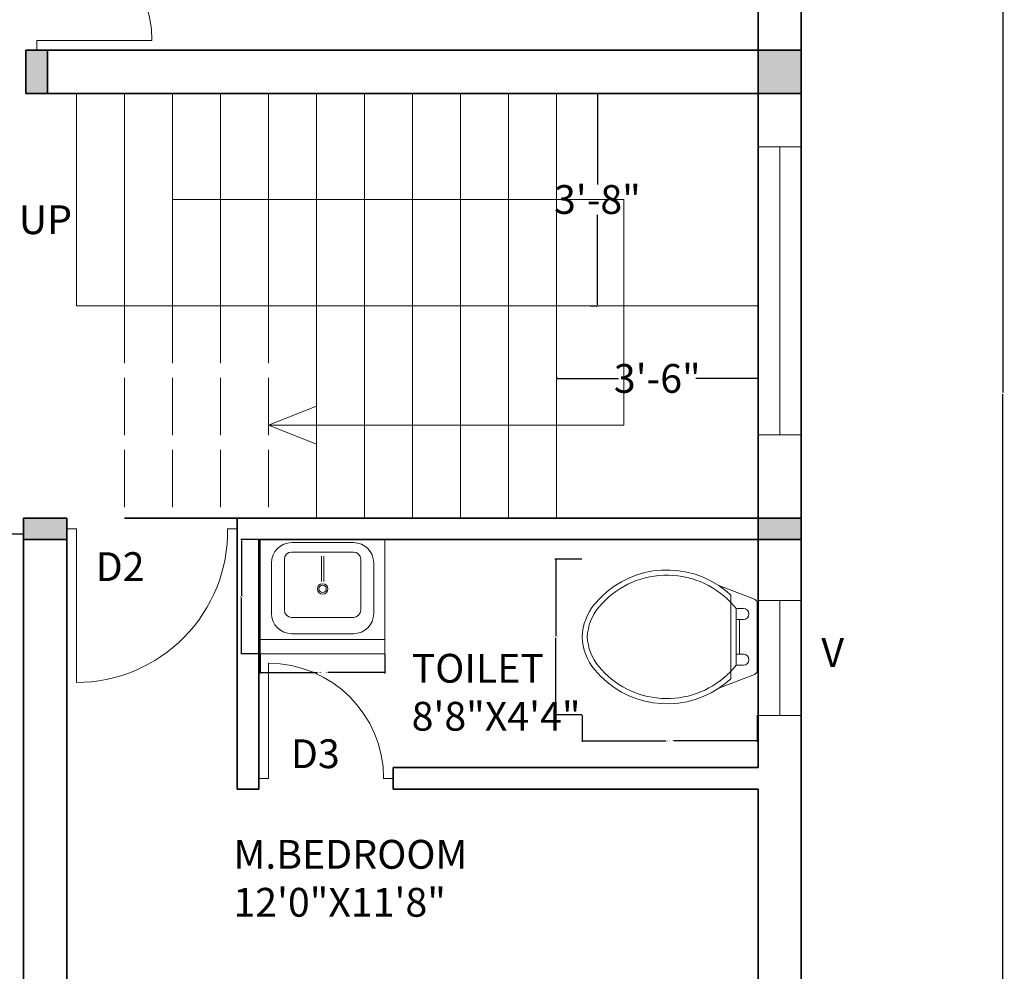
# Model space of a CAD drawing. Units: inches. Extents: x -36302355 to 648, y -221479757 to 75.
# Tile 22 of 37: x 442 to 647, y -469 to -271. Entities that reach past the tile are written whole.
import ezdxf

# ---------------------------------------------------------------- set-up
doc = ezdxf.new("R2010")
doc.units = ezdxf.units.IN
doc.header["$MEASUREMENT"] = 0
doc.linetypes.add('ACAD_ISO02W100', pattern=[15, 12, -3])
for name, color, linetype, lineweight in [('A-ANNO-DIMS', 2, 'Continuous', 18), ('A-ANNO-IDEN', 7, 'Continuous', 18), ('A-ANNO-TEXT', 7, 'Continuous', 18), ('A-AREA-IDEN', 7, 'Continuous', 18), ('A-COLS', 7, 'Continuous', 35), ('A-COLS-PATT', 242, 'Continuous', 13), ('A-DOOR', 4, 'Continuous', 18), ('A-FLOR-FIXT', 9, 'Continuous', 18), ('A-FLOR-STRS', 7, 'Continuous', 18), ('A-FLOR-STRS-HIDN', 7, 'ACAD_ISO02W100', 13), ('A-GLAZ', 142, 'Continuous', 18), ('A-WALL', 7, 'Continuous', 35)]:
    doc.layers.add(name, color=color, linetype=linetype, lineweight=lineweight)
doc.styles.get("Standard").update_dxf_attribs({"font": 'arial.ttf'})
doc.dimstyles.get("Standard").update_dxf_attribs({"dimtxt": 0.18, "dimasz": 0.18, "dimexe": 0.18, "dimexo": 0.0625, "dimgap": 0.09, "dimtad": 0, "dimtih": 1, "dimtoh": 1, "dimdec": 0, "dimzin": 0, "dimdsep": 46, "dimlunit": 3, "dimtxsty": 'Standard', "dimcen": 0.09, "dimadec": 0, "dimazin": 0, "dimtfac": 1, "dimtdec": 0, "dimtofl": 0, "dimtmove": 0, "dimatfit": 3, "dimfxl": 1, "dimtolj": 1, "dimtzin": 0, "dimarcsym": 0})

# ---------------------------------------------------------------- blocks, each defined once
blk = doc.blocks.new('*D5')
at = {"layer": 'A-ANNO-DIMS', "color": 0, "lineweight": -2, "transparency": 16777216}
for p, q in [((401.2, -376.83), (401.2, -378.08)), ((443.2, -376.83), (443.2, -378.08)), ((401.38, -377.9), (414.13, -377.9)), ((443.02, -377.9), (430.26, -377.9))]:
    blk.add_line(p, q, dxfattribs=at)
at = {"layer": 'A-ANNO-DIMS', "color": 0, "transparency": 16777216}
for points in [[(401.38, -377.87), (401.38, -377.93), (401.2, -377.9)], [(443.02, -377.87), (443.02, -377.93), (443.2, -377.9)]]:
    blk.add_solid(points, dxfattribs=at)
at = {"layer": 'Defpoints', "color": 0, "transparency": 16777216}
for p in [(401.2, -376.77), (443.2, -376.77), (443.2, -377.9)]:
    blk.add_point(p, dxfattribs=at)
at = {"layer": 'A-ANNO-DIMS', "color": 0, "transparency": 16777216, "insert": (422.2, -377.9), "char_height": 6, "attachment_point": 5}
blk.add_mtext('\\A1;3\'-6"', dxfattribs=at)
blk = doc.blocks.new('М14 600х655')
for p, q in [((-655, 600), (-655, 0)), ((-655, 600), (-655, 0)), ((-655, 0), (-655, 600)), ((0, 600), (-655, 600)), ((0, 0), (0, 600)), ((0, 525), (-655, 525)), ((-165.1, 494.1), (-489.9, 494.1)), ((-595.8, 388.1), (-595.8, 121.3)), ((-528.4, 370.1), (-528.4, 103.3)), ((-165.4, 408.4), (-490.2, 408.4)), ((-127.2, 103.3), (-127.2, 370.1)), ((-59.2, 121.3), (-59.2, 388.1)), ((-333.5, 87.1), (-333.5, 219.6)), ((-321.5, 87.1), (-321.5, 219.6)), ((-490.2, 65.1), (-165.4, 65.1)), ((-655, 0), (-655, 0)), ((-655, 0), (-655, 0)), ((-655, 0), (0, 0)), ((-655, 0), (0, 0)), ((-489.9, 15.4), (-165.1, 15.4))]:
    blk.add_line(p, q)
for radius in [27.6, 19.3]:
    blk.add_circle((-327.5, 258.9), radius)
for centre, radius, start, end in [((-489.9, 388.1), 105.9, 90, 180), ((-165.1, 388.1), 105.9, 0, 90), ((-490.2, 370.1), 38.2, 90, 180), ((-165.4, 370.1), 38.2, 0, 90), ((-489.9, 121.3), 105.9, 180, 270), ((-165.1, 121.3), 105.9, 270, 0), ((-490.2, 103.3), 38.2, 180, 270), ((-165.4, 103.3), 38.2, 270, 0)]:
    blk.add_arc(centre, radius, start, end)
blk = doc.blocks.new('*D13')
at = {"layer": 'A-ANNO-DIMS', "color": 0, "lineweight": -2, "transparency": 16777216}
for p, q in [((554.2, -345.07), (554.2, -345.6)), ((554.38, -345.42), (567.13, -345.42)), ((596.02, -345.42), (583.26, -345.42)), ((596.2, -345.07), (596.2, -345.6))]:
    blk.add_line(p, q, dxfattribs=at)
at = {"layer": 'A-ANNO-DIMS', "color": 0, "transparency": 16777216}
for points in [[(554.38, -345.39), (554.38, -345.45), (554.2, -345.42)], [(596.02, -345.39), (596.02, -345.45), (596.2, -345.42)]]:
    blk.add_solid(points, dxfattribs=at)
at = {"layer": 'Defpoints', "color": 0, "transparency": 16777216}
for p in [(554.2, -345.01), (596.2, -345.01), (596.2, -345.42)]:
    blk.add_point(p, dxfattribs=at)
at = {"layer": 'A-ANNO-DIMS', "color": 0, "transparency": 16777216, "insert": (575.2, -345.42), "char_height": 6, "attachment_point": 5}
blk.add_mtext('\\A1;3\'-6"', dxfattribs=at)
blk = doc.blocks.new('*D14')
at = {"layer": 'A-ANNO-DIMS', "color": 0, "lineweight": -2, "transparency": 16777216}
for p, q in [((561.2, -286.02), (562.91, -286.02)), ((562.73, -286.2), (562.73, -304.99)), ((562.73, -330.09), (562.73, -311.3)), ((561.2, -330.27), (562.91, -330.27))]:
    blk.add_line(p, q, dxfattribs=at)
at = {"layer": 'A-ANNO-DIMS', "color": 0, "transparency": 16777216}
for points in [[(562.7, -286.2), (562.76, -286.2), (562.73, -286.02)], [(562.7, -330.09), (562.76, -330.09), (562.73, -330.27)]]:
    blk.add_solid(points, dxfattribs=at)
at = {"layer": 'Defpoints', "color": 0, "transparency": 16777216}
for p in [(561.14, -286.02), (562.73, -286.02), (561.14, -330.27)]:
    blk.add_point(p, dxfattribs=at)
at = {"layer": 'A-ANNO-DIMS', "color": 0, "transparency": 16777216, "insert": (562.73, -308.14), "char_height": 6, "attachment_point": 5}
blk.add_mtext('\\A1;3\'-8"', dxfattribs=at)
blk = doc.blocks.new('WC-FLOOR-MOUNT')
for p, q in [((4.02, 15.38), (4.02, 16.49)), ((4.02, 15.38), (4.02, 10.15)), ((4.02, 4.92), (4.02, 10.15)), ((4.02, 3.8), (4.02, 4.92))]:
    blk.add_line(p, q)
for points in [[(4.02, 15.38, -0.448546), (24.05, 14.64, -0.162618), (25.78, 10.15, -0.470877)], [(5.85, 17.93, -0.383919), (24.66, 15.14, -0.163732), (26.58, 10.15, -0.359733)], [(0, 10.15), (0, 15.22, -0.31031), (0.43, 15.85), (5.85, 17.93, -0.209071)], [(4.02, 16.49, -0.040937), (5.85, 17.93, -0.163732)], [(3.22, 14.46, -0.022712), (4.02, 15.38, -0.162618)], [(3.22, 14.46), (2.11, 14.46, 1), (2.11, 12.77), (2.69, 12.77)], [(3.22, 10.15), (3.22, 14.46, -0.476108)], [(0, 10.15), (0, 5.07, 0.31031), (0.43, 4.45), (5.85, 2.37, 0.209071)], [(3.22, 10.15), (3.22, 5.84, 0.022712)], [(4.57, 4.39, 0.431639), (24.05, 5.66, 0.162618), (25.78, 10.15, 0.470877)], [(5.85, 2.37, 0.383919), (24.66, 5.15, 0.163732), (26.58, 10.15, 0.359733)], [(3.22, 5.84), (2.11, 5.84, -1), (2.11, 7.53), (2.69, 7.53)], [(3.22, 5.84, 0.022712), (4.02, 4.92, 0.162618)], [(4.02, 4.92, 0.014165), (4.57, 4.39, 0.162618)], [(4.02, 3.8, 0.040937), (5.85, 2.37, 0.163732)]]:
    blk.add_lwpolyline(points, format="xyb")
for points in [[(2.69, 12.77), (2.69, 7.53)], [(2.69, 12.77), (3.22, 12.77)], [(2.69, 7.53), (3.22, 7.53)]]:
    blk.add_lwpolyline(points)
blk = doc.blocks.new('WIN-60')
for p, q in [((60, 9), (0, 9)), ((0, 9), (0, 0)), ((60, 0), (60, 9)), ((0, 4.5), (60, 4.5)), ((0, 0), (60, 0))]:
    blk.add_line(p, q)
blk = doc.blocks.new('VENT-24')
for p, q in [((0, 0), (0, 24)), ((0, 24), (9, 24)), ((4.5, 24), (4.5, 0)), ((9, 24), (9, 0)), ((9, 0), (0, 0))]:
    blk.add_line(p, q)
blk = doc.blocks.new('DOOR-SWING-24')
for p, q in [((0, 26), (0, 28)), ((0, 0), (0, 2)), ((0, 2), (24, 2))]:
    blk.add_line(p, q)
blk.add_arc((0, 2), 24, 0, 90)
blk = doc.blocks.new('*D29')
at = {"layer": 'A-ANNO-DIMS', "color": 0, "lineweight": -2, "transparency": 16777216}
for p, q in [((492.52, -402.87), (492.52, -406.88)), ((518.48, -402.87), (518.48, -406.88)), ((492.7, -406.7), (504.45, -406.7)), ((518.3, -406.7), (506.55, -406.7))]:
    blk.add_line(p, q, dxfattribs=at)
at = {"layer": 'A-ANNO-DIMS', "color": 0, "transparency": 16777216}
for points in [[(492.7, -406.67), (492.7, -406.73), (492.52, -406.7)], [(518.3, -406.67), (518.3, -406.73), (518.48, -406.7)]]:
    blk.add_solid(points, dxfattribs=at)
at = {"layer": 'Defpoints', "color": 0, "transparency": 16777216}
for p in [(492.52, -402.81), (518.48, -402.81), (518.48, -406.7)]:
    blk.add_point(p, dxfattribs=at)
at = {"layer": 'A-ANNO-DIMS', "color": 0, "transparency": 16777216, "insert": (505.5, -406.7), "char_height": 0.18, "attachment_point": 5}
blk.add_mtext('\\A1;BASIN 2\'-2" TYP.', dxfattribs=at)
blk = doc.blocks.new('*D30')
at = {"layer": 'A-ANNO-DIMS', "color": 0, "lineweight": -2, "transparency": 16777216}
for p, q in [((492.45, -379.02), (488.44, -379.02)), ((488.62, -379.2), (488.62, -390.73)), ((488.62, -402.63), (488.62, -391.09)), ((492.45, -402.81), (488.44, -402.81))]:
    blk.add_line(p, q, dxfattribs=at)
at = {"layer": 'A-ANNO-DIMS', "color": 0, "transparency": 16777216}
for points in [[(488.59, -379.2), (488.65, -379.2), (488.62, -379.02)], [(488.59, -402.63), (488.65, -402.63), (488.62, -402.81)]]:
    blk.add_solid(points, dxfattribs=at)
at = {"layer": 'Defpoints', "color": 0, "transparency": 16777216}
for p in [(492.52, -379.02), (488.62, -402.81), (492.52, -402.81)]:
    blk.add_point(p, dxfattribs=at)
at = {"layer": 'A-ANNO-DIMS', "color": 0, "transparency": 16777216, "insert": (488.62, -390.91), "char_height": 0.18, "attachment_point": 5}
blk.add_mtext('\\A1;2\'-0" TYP.', dxfattribs=at)
blk = doc.blocks.new('*D41')
at = {"layer": 'A-ANNO-DIMS', "color": 0, "lineweight": -2, "transparency": 16777216}
for p, q in [((559.53, -415.56), (559.53, -421.15)), ((596.04, -415.56), (596.04, -421.15)), ((559.71, -420.97), (577, -420.97)), ((595.86, -420.97), (578.57, -420.97))]:
    blk.add_line(p, q, dxfattribs=at)
at = {"layer": 'A-ANNO-DIMS', "color": 0, "transparency": 16777216}
for points in [[(559.71, -420.94), (559.71, -421), (559.53, -420.97)], [(595.86, -420.94), (595.86, -421), (596.04, -420.97)]]:
    blk.add_solid(points, dxfattribs=at)
at = {"layer": 'Defpoints', "color": 0, "transparency": 16777216}
for p in [(559.53, -415.5), (596.04, -415.5), (559.53, -420.97)]:
    blk.add_point(p, dxfattribs=at)
at = {"layer": 'A-ANNO-DIMS', "color": 0, "transparency": 16777216, "insert": (577.78, -420.97), "char_height": 0.18, "attachment_point": 5}
blk.add_mtext('\\A1;WC 3\'-0 1/2"', dxfattribs=at)
blk = doc.blocks.new('*D42')
at = {"layer": 'A-ANNO-DIMS', "color": 0, "lineweight": -2, "transparency": 16777216}
for p, q in [((559.47, -383.06), (553.87, -383.06)), ((554.05, -383.24), (554.05, -399.1)), ((554.05, -415.32), (554.05, -399.46)), ((559.47, -415.5), (553.87, -415.5))]:
    blk.add_line(p, q, dxfattribs=at)
at = {"layer": 'A-ANNO-DIMS', "color": 0, "transparency": 16777216}
for points in [[(554.02, -383.24), (554.08, -383.24), (554.05, -383.06)], [(554.02, -415.32), (554.08, -415.32), (554.05, -415.5)]]:
    blk.add_solid(points, dxfattribs=at)
at = {"layer": 'Defpoints', "color": 0, "transparency": 16777216}
for p in [(554.05, -383.06), (559.53, -383.06), (559.53, -415.5)]:
    blk.add_point(p, dxfattribs=at)
at = {"layer": 'A-ANNO-DIMS', "color": 0, "transparency": 16777216, "insert": (554.05, -399.28), "char_height": 0.18, "attachment_point": 5}
blk.add_mtext('\\A1;2\'-8 1/2"', dxfattribs=at)
blk = doc.blocks.new('*D57')
at = {"layer": 'A-ANNO-DIMS', "color": 0, "lineweight": -2, "transparency": 16777216}
for p, q in [((605.26, 24.98), (647.33, 24.98)), ((647.15, 24.8), (647.15, -348.34)), ((647.15, -721.84), (647.15, -348.7)), ((605.26, -722.02), (647.33, -722.02))]:
    blk.add_line(p, q, dxfattribs=at)
at = {"layer": 'A-ANNO-DIMS', "color": 0, "transparency": 16777216}
for points in [[(647.12, 24.8), (647.18, 24.8), (647.15, 24.98)], [(647.12, -721.84), (647.18, -721.84), (647.15, -722.02)]]:
    blk.add_solid(points, dxfattribs=at)
at = {"layer": 'Defpoints', "color": 0, "transparency": 16777216}
for p in [(605.2, 24.98), (605.2, -722.02), (647.15, -722.02)]:
    blk.add_point(p, dxfattribs=at)
at = {"layer": 'A-ANNO-DIMS', "color": 0, "transparency": 16777216, "insert": (647.15, -348.52), "char_height": 0.18, "attachment_point": 5}
blk.add_mtext('\\A1;62\'-3"', dxfattribs=at)

msp = doc.modelspace()

# ---------------------------------------------------------------- hatches: boundary and pattern name
at = {"layer": 'A-COLS-PATT'}
h = msp.add_hatch(color=256, dxfattribs=at)
h.dxf.hatch_style = 1
h.paths.add_polyline_path([(145.2, 24.98), (145.2, 15.98), (154.2, 15.98), (154.2, 24.98)])
h.paths.add_polyline_path([(247.2, 15.98), (247.2, 24.98), (238.2, 24.98), (238.2, 15.98)])
h.paths.add_polyline_path([(387.64, 15.98), (395.7, 15.98), (395.7, 24.98), (387.64, 24.98)])
h.paths.add_polyline_path([(451.26, 24.98), (443.7, 24.98), (443.7, 15.98), (451.26, 15.98)])
h.paths.add_polyline_path([(596.2, 15.98), (605.2, 15.98), (605.2, 24.98), (596.2, 24.98)])
h.paths.add_polyline_path([(238.2, -122.02), (238.2, -131.02), (247.2, -131.02), (247.2, -122.02)])
h.paths.add_polyline_path([(395.7, -122.02), (387.46, -122.02), (387.46, -131.02), (395.7, -131.02)])
h.paths.add_polyline_path([(448.2, -131.02), (453.73, -131.02), (453.73, -122.02), (443.7, -122.02), (443.7, -131.02)])
h.paths.add_polyline_path([(596.2, -131.02), (605.2, -131.02), (605.2, -122.02), (596.2, -122.02)])
h.paths.add_polyline_path([(145.2, -176.97), (154.2, -176.97), (154.2, -167.02), (145.2, -167.02)])
h.paths.add_polyline_path([(314.2, -176.97), (323.2, -176.97), (323.2, -167.02), (314.2, -167.02)])
h.paths.add_polyline_path([(154.2, -314.02), (154.2, -309.52), (145.2, -309.52), (145.2, -314.02)])
h.paths.add_polyline_path([(314.2, -309.52), (314.2, -318.52), (323.2, -318.52), (323.2, -309.52)])
h.paths.add_polyline_path([(448.2, -277.02), (443.7, -277.02), (443.7, -286.02), (448.2, -286.02)])
h.paths.add_polyline_path([(283.2, -370.02), (274.2, -370.02), (274.2, -379.02), (283.2, -379.02), (283.2, -374.52)])
h.paths.add_polyline_path([(154.2, -370.02), (145.2, -370.02), (145.2, -379.02), (154.2, -379.02)])
h.paths.add_polyline_path([(443.2, -374.52), (443.2, -379.02), (452.2, -379.02), (452.2, -374.52)])
h.paths.add_polyline_path([(145.2, -580.02), (154.2, -580.02), (154.2, -571.02), (145.2, -571.02)])
h.paths.add_polyline_path([(274.2, -571.02), (274.2, -580.02), (283.2, -580.02), (283.2, -571.02)])
h.paths.add_polyline_path([(443.2, -580.02), (452.2, -580.02), (452.2, -571.02), (443.2, -571.02)])
h = msp.add_hatch(color=256, dxfattribs=at)
h.dxf.hatch_style = 1
h.paths.add_polyline_path([(596.2, -277.02), (596.2, -286.02), (605.2, -286.02), (605.2, -277.02)])
h = msp.add_hatch(color=256, dxfattribs=at)
h.dxf.hatch_style = 1
h.paths.add_polyline_path([(605.2, -571.02), (596.2, -571.02), (596.2, -580.02), (605.2, -580.02)])
h.paths.add_polyline_path([(605.2, -374.52), (596.2, -374.52), (596.2, -379.02), (605.2, -379.02)])

# ---------------------------------------------------------------- linework, layer by layer
at = {"layer": 'A-COLS'}
for p, q in [((443.7, -277.02), (443.7, -286.02)), ((448.2, -277.02), (448.2, -286.02)), ((443.2, -374.52), (452.2, -374.52)), ((443.2, -379.02), (452.2, -379.02))]:
    msp.add_line(p, q, dxfattribs=at)
at = {"layer": 'A-DOOR'}
for p, q in [((452.2, -376.77), (454.2, -376.77)), ((454.2, -376.77), (454.2, -408.77)), ((487.7, -376.77), (485.7, -376.77))]:
    msp.add_line(p, q, dxfattribs=at)
msp.add_arc((454.2, -377.27), 31.5, 270, 0.9023, dxfattribs=at)
at = {"layer": 'A-FLOR-STRS'}
for p, q in [((454.2, -286.02), (454.2, -330.27)), ((464.2, -286.02), (464.2, -330.27)), ((474.2, -286.02), (474.2, -330.27)), ((484.2, -286.02), (484.2, -330.27)), ((494.2, -286.02), (494.2, -330.27)), ((504.2, -286.02), (504.2, -374.52)), ((514.2, -286.02), (514.2, -374.52)), ((524.2, -286.02), (524.2, -374.52)), ((534.2, -286.02), (534.2, -374.52)), ((544.2, -286.02), (544.2, -374.52)), ((554.2, -286.02), (554.2, -374.52)), ((474.2, -308.14), (568.21, -308.14)), ((568.21, -308.14), (568.21, -355.15)), ((454.2, -330.27), (596.2, -330.27)), ((494.2, -355.15), (504.2, -351.19)), ((568.21, -355.15), (494.2, -355.15)), ((494.2, -355.15), (504.2, -359.11))]:
    msp.add_line(p, q, dxfattribs=at)
at = {"layer": 'A-FLOR-STRS-HIDN'}
for p, q in [((464.2, -330.27), (464.2, -374.52)), ((474.2, -330.27), (474.2, -374.52)), ((484.2, -330.27), (484.2, -374.52)), ((494.2, -330.27), (494.2, -374.52))]:
    msp.add_line(p, q, dxfattribs=at)
at = {"layer": 'A-WALL'}
for p, q in [((596.2, 24.98), (596.2, -426.52)), ((605.2, 24.98), (605.2, -722.02)), ((443.7, -277.02), (605.2, -277.02)), ((443.7, -286.02), (605.2, -286.02)), ((443.2, -374.52), (443.2, -580.02)), ((452.2, -374.52), (452.2, -580.02)), ((464.2, -374.52), (605.2, -374.52)), ((487.7, -374.52), (487.7, -426.52)), ((492.2, -379.02), (605.2, -379.02)), ((492.2, -379.02), (492.2, -426.52)), ((487.7, -426.52), (487.7, -431.02)), ((492.2, -426.52), (492.2, -431.02)), ((520.2, -428.77), (520.2, -426.52)), ((520.2, -426.52), (596.2, -426.52)), ((520.2, -428.77), (520.2, -431.02)), ((487.7, -431.02), (492.2, -431.02)), ((520.2, -431.02), (596.2, -431.02)), ((596.2, -431.02), (596.2, -722.02))]:
    msp.add_line(p, q, dxfattribs=at)

# ---------------------------------------------------------------- block references
at = {"layer": 'A-DOOR'}
msp.add_blockref('DOOR-SWING-24', (445.95, -277.02), dxfattribs=at)
at = {"layer": 'A-DOOR', "extrusion": (0, 0, -1), "zscale": -1, "rotation": 90}
msp.add_blockref('DOOR-SWING-24', (-492.2, -428.77), dxfattribs=at)
at = {"layer": 'A-FLOR-FIXT', "xscale": -0.0396455158158922, "yscale": 0.0396455158158922, "zscale": 0.0396455158158922, "rotation": 180}
msp.add_blockref('М14 600х655', (518.48, -379.02), dxfattribs=at)
at = {"layer": 'A-FLOR-FIXT', "extrusion": (0, 0, -1), "xscale": 1.373542475262903, "yscale": 1.373542475262903, "zscale": -1}
msp.add_blockref('WC-FLOOR-MOUNT', (-596.04, -413.22), dxfattribs=at)
at = {"layer": 'A-GLAZ', "extrusion": (0, 0, -1), "zscale": -1, "rotation": 90}
msp.add_blockref('WIN-60', (-596.2, -357.19), dxfattribs=at)
at = {"layer": 'A-GLAZ'}
msp.add_blockref('VENT-24', (596.2, -415.69), dxfattribs=at)

# ---------------------------------------------------------------- texts
at = {"layer": 'A-ANNO-IDEN', "char_height": 6, "attachment_point": 1}
for s, insert in [('D2', (458.22, -381.64)), ('V', (609.38, -399.54)), ('D3', (498.89, -420.63))]:
    msp.add_mtext(s, dxfattribs=dict(at, insert=insert))
at = {"layer": 'A-ANNO-TEXT', "insert": (442.21, -309.35), "char_height": 6, "attachment_point": 1}
msp.add_mtext('UP', dxfattribs=at)
at = {"layer": 'A-AREA-IDEN', "char_height": 6, "attachment_point": 1}
for s, insert in [('TOILET\\P8\'8"X4\'4"', (524.04, -402.82)), ('M.BEDROOM\\P12\'0"X11\'8"', (486.91, -441.59))]:
    msp.add_mtext(s, dxfattribs=dict(at, insert=insert))

# ---------------------------------------------------------------- dimensions: what is measured, and where the dimension line sits
at = {"layer": 'A-ANNO-DIMS'}
for base, p1, p2, override, picture, middle in [((647.15, -722.02), (605.2, 24.98), (605.2, -722.02), {"dimdec": 1, "dimlfac": 1, "dimrnd": 0, "dimzin": 1, "dimdsep": 46, "dimlunit": 4, "dimfrac": 2}, '*D57', (647.15, -348.52)), ((562.73, -286.02), (561.14, -330.27), (561.14, -286.02), {"dimtxt": 6, "dimclrd": 0, "dimclre": 0, "dimclrt": 0}, '*D14', (562.73, -308.14)), ((554.05, -383.06), (559.53, -415.5), (559.53, -383.06), {"dimdec": 1, "dimlfac": 1, "dimrnd": 0, "dimzin": 1, "dimdsep": 46, "dimlunit": 4, "dimfrac": 2}, '*D42', (554.05, -399.28))]:
    dim = msp.add_linear_dim(base=base, p1=p1, p2=p2, angle=90, dimstyle='Standard', override=override, dxfattribs=at)
    dim.commit()
    dim.dimension.update_dxf_attribs({"geometry": picture, "text_midpoint": middle})
for base, p1, p2, picture, middle in [((596.2, -345.42), (554.2, -345.01), (596.2, -345.01), '*D13', (575.2, -345.42)), ((443.2, -377.9), (401.2, -376.77), (443.2, -376.77), '*D5', (422.2, -377.9))]:
    dim = msp.add_linear_dim(base=base, p1=p1, p2=p2, dimstyle='Standard', override={"dimtxt": 6, "dimclrd": 0, "dimclre": 0, "dimclrt": 0}, dxfattribs=at)
    dim.commit()
    dim.dimension.update_dxf_attribs({"geometry": picture, "text_midpoint": middle})
for base, p1, p2, angle, text, picture, middle in [((488.62, -402.81), (492.52, -379.02), (492.52, -402.81), 270, '<> TYP.', '*D30', (488.62, -390.91)), ((559.53, -420.97), (596.04, -415.5), (559.53, -415.5), 180, 'WC <>', '*D41', (577.78, -420.97))]:
    dim = msp.add_linear_dim(base=base, p1=p1, p2=p2, angle=angle, text=text, dimstyle='Standard', override={"dimdec": 1, "dimlfac": 1, "dimrnd": 0, "dimzin": 1, "dimdsep": 46, "dimlunit": 4, "dimfrac": 2}, dxfattribs=at)
    dim.commit()
    dim.dimension.update_dxf_attribs({"geometry": picture, "text_midpoint": middle})
dim = msp.add_linear_dim(base=(518.48, -406.7), p1=(492.52, -402.81), p2=(518.48, -402.81), text='BASIN <> TYP.', dimstyle='Standard', override={"dimdec": 1, "dimlfac": 1, "dimrnd": 0, "dimzin": 1, "dimdsep": 46, "dimlunit": 4, "dimfrac": 2}, dxfattribs=at)
dim.commit()
dim.dimension.update_dxf_attribs({"geometry": '*D29', "text_midpoint": (505.5, -406.7)})

doc.saveas('drawing.dxf')
